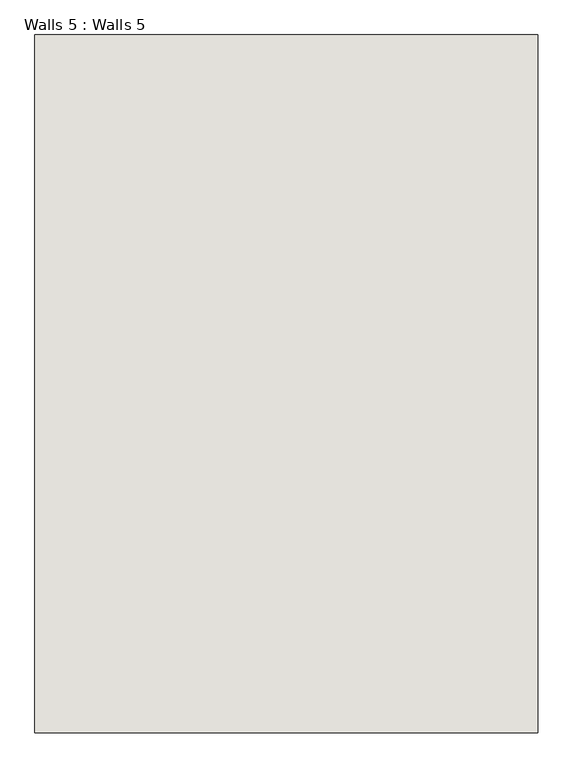
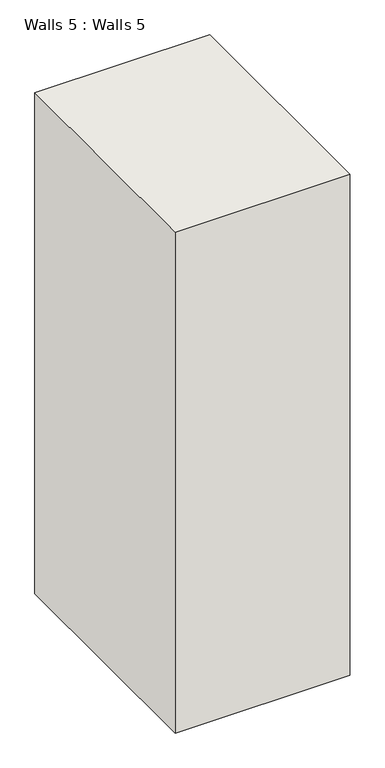
"""IFC4 building model written with IfcOpenShell, lengths in millimetres: wall geometry, Walls 5 : Walls 5."""

from ifc_helpers import new_model, si_unit, frame, origin, place, context, project, spatial, polyline, outline, extrude, source, transform, mapped, element, save


def walls_5_walls_5_067f5539(model_context):
    return source(origin(), model_context, "Body", "SweptSolid", [
        extrude(outline(polyline([(-12118.8440117, 9681.6609482), (-12118.8440117, 11358.0609482), (-10910.9897233, 11358.0609482), (-10910.9897233, 9681.6609482), (-12118.8440117, 9681.6609482)])), frame((0.0, 0.0, 7010.4), z_axis=(0.0, 0.0, 1.0), x_axis=(1.0, 0.0, 0.0)), (0.0, 0.0, 1.0), 3657.6),
    ])


if __name__ == "__main__":
    model = new_model("IFC4")
    model_context = context("Model", 3, world=origin())
    ifc_project = project(units=[si_unit("LENGTHUNIT", "METRE", prefix="MILLI")], contexts=[model_context])
    site = spatial("IfcSite", under=ifc_project)
    building = spatial("IfcBuilding", under=site)
    placement = place(None, origin())
    walls_5_walls_5_shape = walls_5_walls_5_067f5539(model_context)
    element("IfcWall", 1, ObjectType="Walls 5 : Walls 5", at=placement, inside=building, context=model_context, shape_type="MappedRepresentation", body=[
        mapped(walls_5_walls_5_shape, transform((0.0, 0.0, 0.0), x_axis=(1.0, 0.0, 0.0), y_axis=(0.0, 1.0, 0.0), z_axis=(0.0, 0.0, 1.0))),
    ])
    save(model, "model.ifc")

# Revit data of these elements
# Element 1 (IfcWall, "Walls 5 : Walls 5")
#   Materials on its faces: "Default Wall"
# Materials
#   "Default Wall": colour RGB 128 128 128, transparency 0
